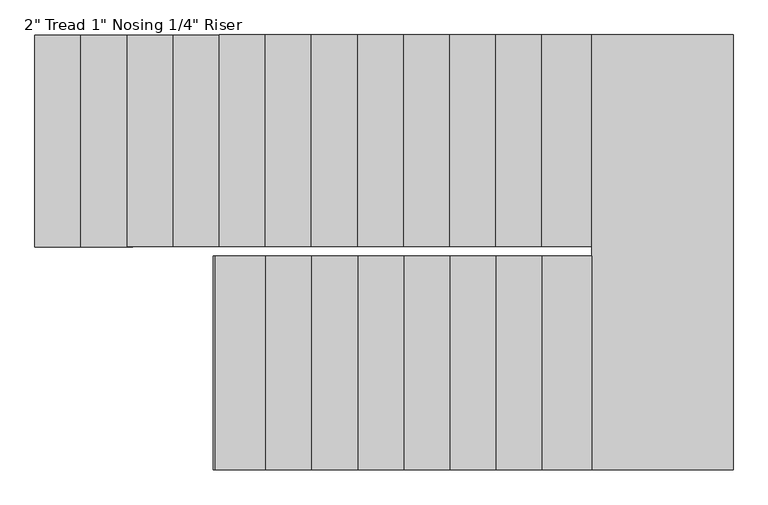
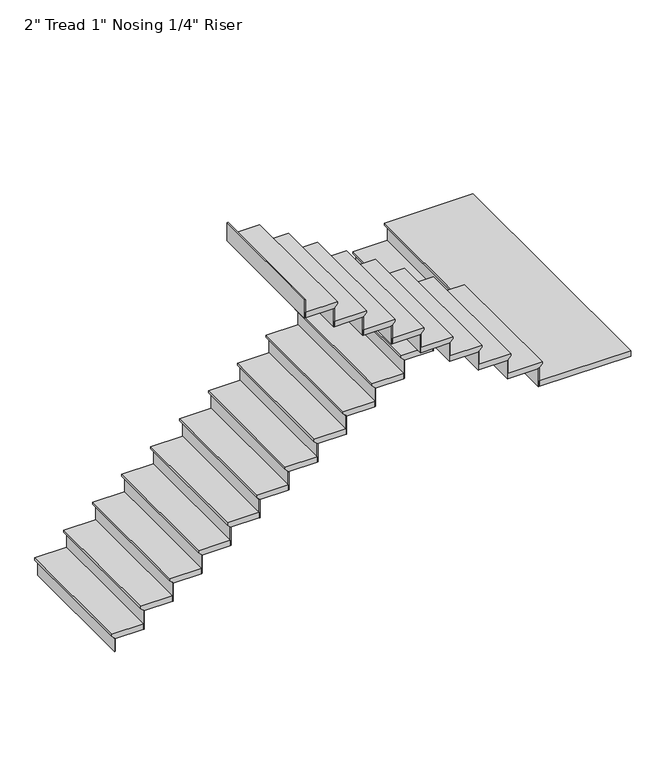
"""IFC4 building model written with IfcOpenShell, lengths in millimetres: stair flight geometry."""

from ifc_helpers import new_model, si_unit, origin, place, context, project, spatial, faceted_brep, source, transform, mapped, element, save


def stair_flight_20087966(model_context):
    return source(origin(), model_context, "Body", "Brep", [
        faceted_brep([(1811.8890963, 296.3962251, 150.2833333), (1811.8890963, 296.3962251, 169.3333333), (1811.8890963, 1464.7962251, 169.3333333), (1811.8890963, 1464.7962251, 150.2833333), (1837.2890963, 296.3962251, 124.8833333), (1837.2890963, 1464.7962251, 124.8833333), (2091.2890963, 296.3962251, 169.3333333), (2091.2890963, 1464.7962251, 169.3333333), (1837.2890963, 1464.7962251, 118.5333333), (2091.2890963, 1464.7962251, 118.5333333), (2091.2890963, 296.3962251, 118.5333333), (1837.2890963, 296.3962251, 118.5333333)], [[[0, 1, 2, 3]], [[4, 0, 3, 5]], [[2, 1, 6, 7]], [[8, 9, 10, 11]], [[2, 7, 9, 8, 5, 3]], [[8, 11, 4, 5]], [[6, 1, 0, 4, 11, 10]], [[7, 6, 10, 9]]]),
        faceted_brep([(1837.2890963, 296.3962251, 118.5333333), (1837.2890963, 296.3962251, 0.0), (1843.6390963, 296.3962251, 0.0), (1843.6390963, 296.3962251, 118.5333333), (1837.2890963, 1464.7962251, 118.5333333), (1843.6390963, 1464.7962251, 118.5333333), (1843.6390963, 1464.7962251, 0.0), (1837.2890963, 1464.7962251, 0.0)], [[[0, 1, 2, 3]], [[4, 5, 6, 7]], [[1, 0, 4, 7]], [[2, 1, 7, 6]], [[3, 2, 6, 5]], [[0, 3, 5, 4]]]),
        faceted_brep([(2091.2890963, 296.3962251, 287.8666667), (2091.2890963, 296.3962251, 118.5333333), (2097.6390963, 296.3962251, 118.5333333), (2097.6390963, 296.3962251, 287.8666667), (2091.2890963, 1464.7962251, 287.8666667), (2097.6390963, 1464.7962251, 287.8666667), (2097.6390963, 1464.7962251, 118.5333333), (2091.2890963, 1464.7962251, 118.5333333)], [[[0, 1, 2, 3]], [[4, 5, 6, 7]], [[1, 0, 4, 7]], [[2, 1, 7, 6]], [[3, 2, 6, 5]], [[0, 3, 5, 4]]]),
        faceted_brep([(2065.8890963, 1464.7962251, 338.6666667), (2065.8890963, 296.3962251, 338.6666667), (2345.2890963, 296.3962251, 338.6666667), (2345.2890963, 1464.7962251, 338.6666667), (2091.2890963, 1464.7962251, 287.8666667), (2345.2890963, 1464.7962251, 287.8666667), (2345.2890963, 296.3962251, 287.8666667), (2091.2890963, 296.3962251, 287.8666667), (2091.2890963, 1464.7962251, 294.2166667), (2065.8890963, 1464.7962251, 319.6166667), (2091.2890963, 296.3962251, 294.2166667), (2065.8890963, 296.3962251, 319.6166667)], [[[0, 1, 2, 3]], [[4, 5, 6, 7]], [[0, 3, 5, 4, 8, 9]], [[4, 7, 10, 8]], [[2, 1, 11, 10, 7, 6]], [[3, 2, 6, 5]], [[11, 1, 0, 9]], [[10, 11, 9, 8]]]),
        faceted_brep([(2345.2890963, 296.3962251, 457.2), (2345.2890963, 296.3962251, 287.8666667), (2351.6390963, 296.3962251, 287.8666667), (2351.6390963, 296.3962251, 457.2), (2345.2890963, 1464.7962251, 457.2), (2351.6390963, 1464.7962251, 457.2), (2351.6390963, 1464.7962251, 287.8666667), (2345.2890963, 1464.7962251, 287.8666667)], [[[0, 1, 2, 3]], [[4, 5, 6, 7]], [[1, 0, 4, 7]], [[2, 1, 7, 6]], [[3, 2, 6, 5]], [[0, 3, 5, 4]]]),
        faceted_brep([(2319.8890963, 1464.7962251, 508.0), (2319.8890963, 296.3962251, 508.0), (2599.2890963, 296.3962251, 508.0), (2599.2890963, 1464.7962251, 508.0), (2345.2890963, 1464.7962251, 457.2), (2599.2890963, 1464.7962251, 457.2), (2599.2890963, 296.3962251, 457.2), (2345.2890963, 296.3962251, 457.2), (2345.2890963, 1464.7962251, 463.55), (2319.8890963, 1464.7962251, 488.95), (2345.2890963, 296.3962251, 463.55), (2319.8890963, 296.3962251, 488.95)], [[[0, 1, 2, 3]], [[4, 5, 6, 7]], [[0, 3, 5, 4, 8, 9]], [[4, 7, 10, 8]], [[2, 1, 11, 10, 7, 6]], [[3, 2, 6, 5]], [[11, 1, 0, 9]], [[10, 11, 9, 8]]]),
        faceted_brep([(2599.2890963, 296.3962251, 626.5333333), (2599.2890963, 296.3962251, 457.2), (2605.6390963, 296.3962251, 457.2), (2605.6390963, 296.3962251, 626.5333333), (2599.2890963, 1464.7962251, 626.5333333), (2605.6390963, 1464.7962251, 626.5333333), (2605.6390963, 1464.7962251, 457.2), (2599.2890963, 1464.7962251, 457.2)], [[[0, 1, 2, 3]], [[4, 5, 6, 7]], [[1, 0, 4, 7]], [[2, 1, 7, 6]], [[3, 2, 6, 5]], [[0, 3, 5, 4]]]),
        faceted_brep([(2573.8890963, 1464.7962251, 677.3333333), (2573.8890963, 296.3962251, 677.3333333), (2853.2890963, 296.3962251, 677.3333333), (2853.2890963, 1464.7962251, 677.3333333), (2599.2890963, 1464.7962251, 626.5333333), (2853.2890963, 1464.7962251, 626.5333333), (2853.2890963, 296.3962251, 626.5333333), (2599.2890963, 296.3962251, 626.5333333), (2599.2890963, 1464.7962251, 632.8833333), (2573.8890963, 1464.7962251, 658.2833333), (2599.2890963, 296.3962251, 632.8833333), (2573.8890963, 296.3962251, 658.2833333)], [[[0, 1, 2, 3]], [[4, 5, 6, 7]], [[0, 3, 5, 4, 8, 9]], [[4, 7, 10, 8]], [[2, 1, 11, 10, 7, 6]], [[3, 2, 6, 5]], [[11, 1, 0, 9]], [[10, 11, 9, 8]]]),
        faceted_brep([(2853.2890963, 296.3962251, 795.8666667), (2853.2890963, 296.3962251, 626.5333333), (2859.6390963, 296.3962251, 626.5333333), (2859.6390963, 296.3962251, 795.8666667), (2853.2890963, 1464.7962251, 795.8666667), (2859.6390963, 1464.7962251, 795.8666667), (2859.6390963, 1464.7962251, 626.5333333), (2853.2890963, 1464.7962251, 626.5333333)], [[[0, 1, 2, 3]], [[4, 5, 6, 7]], [[1, 0, 4, 7]], [[2, 1, 7, 6]], [[3, 2, 6, 5]], [[0, 3, 5, 4]]]),
        faceted_brep([(2827.8890963, 1464.7962251, 846.6666667), (2827.8890963, 296.3962251, 846.6666667), (3107.2890963, 296.3962251, 846.6666667), (3107.2890963, 1464.7962251, 846.6666667), (2853.2890963, 1464.7962251, 795.8666667), (3107.2890963, 1464.7962251, 795.8666667), (3107.2890963, 296.3962251, 795.8666667), (2853.2890963, 296.3962251, 795.8666667), (2853.2890963, 1464.7962251, 802.2166667), (2827.8890963, 1464.7962251, 827.6166667), (2853.2890963, 296.3962251, 802.2166667), (2827.8890963, 296.3962251, 827.6166667)], [[[0, 1, 2, 3]], [[4, 5, 6, 7]], [[0, 3, 5, 4, 8, 9]], [[4, 7, 10, 8]], [[2, 1, 11, 10, 7, 6]], [[3, 2, 6, 5]], [[11, 1, 0, 9]], [[10, 11, 9, 8]]]),
        faceted_brep([(3107.2890963, 296.3962251, 965.2), (3107.2890963, 296.3962251, 795.8666667), (3113.6390963, 296.3962251, 795.8666667), (3113.6390963, 296.3962251, 965.2), (3107.2890963, 1464.7962251, 965.2), (3113.6390963, 1464.7962251, 965.2), (3113.6390963, 1464.7962251, 795.8666667), (3107.2890963, 1464.7962251, 795.8666667)], [[[0, 1, 2, 3]], [[4, 5, 6, 7]], [[1, 0, 4, 7]], [[2, 1, 7, 6]], [[3, 2, 6, 5]], [[0, 3, 5, 4]]]),
        faceted_brep([(3081.8890963, 1464.7962251, 1016.0), (3081.8890963, 296.3962251, 1016.0), (3361.2890963, 296.3962251, 1016.0), (3361.2890963, 1464.7962251, 1016.0), (3107.2890963, 1464.7962251, 965.2), (3361.2890963, 1464.7962251, 965.2), (3361.2890963, 296.3962251, 965.2), (3107.2890963, 296.3962251, 965.2), (3107.2890963, 1464.7962251, 971.55), (3081.8890963, 1464.7962251, 996.95), (3107.2890963, 296.3962251, 971.55), (3081.8890963, 296.3962251, 996.95)], [[[0, 1, 2, 3]], [[4, 5, 6, 7]], [[0, 3, 5, 4, 8, 9]], [[4, 7, 10, 8]], [[2, 1, 11, 10, 7, 6]], [[3, 2, 6, 5]], [[11, 1, 0, 9]], [[10, 11, 9, 8]]]),
        faceted_brep([(3361.2890963, 296.3962251, 1134.5333333), (3361.2890963, 296.3962251, 965.2), (3367.6390963, 296.3962251, 965.2), (3367.6390963, 296.3962251, 1134.5333333), (3361.2890963, 1464.7962251, 1134.5333333), (3367.6390963, 1464.7962251, 1134.5333333), (3367.6390963, 1464.7962251, 965.2), (3361.2890963, 1464.7962251, 965.2)], [[[0, 1, 2, 3]], [[4, 5, 6, 7]], [[1, 0, 4, 7]], [[2, 1, 7, 6]], [[3, 2, 6, 5]], [[0, 3, 5, 4]]]),
        faceted_brep([(3335.8890963, 1464.7962251, 1185.3333333), (3335.8890963, 296.3962251, 1185.3333333), (3615.2890963, 296.3962251, 1185.3333333), (3615.2890963, 1464.7962251, 1185.3333333), (3361.2890963, 1464.7962251, 1134.5333333), (3615.2890963, 1464.7962251, 1134.5333333), (3615.2890963, 296.3962251, 1134.5333333), (3361.2890963, 296.3962251, 1134.5333333), (3361.2890963, 1464.7962251, 1140.8833333), (3335.8890963, 1464.7962251, 1166.2833333), (3361.2890963, 296.3962251, 1140.8833333), (3335.8890963, 296.3962251, 1166.2833333)], [[[0, 1, 2, 3]], [[4, 5, 6, 7]], [[0, 3, 5, 4, 8, 9]], [[4, 7, 10, 8]], [[2, 1, 11, 10, 7, 6]], [[3, 2, 6, 5]], [[11, 1, 0, 9]], [[10, 11, 9, 8]]]),
        faceted_brep([(3615.2890963, 296.3962251, 1303.8666667), (3615.2890963, 296.3962251, 1134.5333333), (3621.6390963, 296.3962251, 1134.5333333), (3621.6390963, 296.3962251, 1303.8666667), (3615.2890963, 1464.7962251, 1303.8666667), (3621.6390963, 1464.7962251, 1303.8666667), (3621.6390963, 1464.7962251, 1134.5333333), (3615.2890963, 1464.7962251, 1134.5333333)], [[[0, 1, 2, 3]], [[4, 5, 6, 7]], [[1, 0, 4, 7]], [[2, 1, 7, 6]], [[3, 2, 6, 5]], [[0, 3, 5, 4]]]),
        faceted_brep([(3589.8890963, 1464.7962251, 1354.6666667), (3589.8890963, 296.3962251, 1354.6666667), (3869.2890963, 296.3962251, 1354.6666667), (3869.2890963, 1464.7962251, 1354.6666667), (3615.2890963, 1464.7962251, 1303.8666667), (3869.2890963, 1464.7962251, 1303.8666667), (3869.2890963, 296.3962251, 1303.8666667), (3615.2890963, 296.3962251, 1303.8666667), (3615.2890963, 1464.7962251, 1310.2166667), (3589.8890963, 1464.7962251, 1335.6166667), (3615.2890963, 296.3962251, 1310.2166667), (3589.8890963, 296.3962251, 1335.6166667)], [[[0, 1, 2, 3]], [[4, 5, 6, 7]], [[0, 3, 5, 4, 8, 9]], [[4, 7, 10, 8]], [[2, 1, 11, 10, 7, 6]], [[3, 2, 6, 5]], [[11, 1, 0, 9]], [[10, 11, 9, 8]]]),
        faceted_brep([(3869.2890963, 296.3962251, 1473.2), (3869.2890963, 296.3962251, 1303.8666667), (3875.6390963, 296.3962251, 1303.8666667), (3875.6390963, 296.3962251, 1473.2), (3869.2890963, 1464.7962251, 1473.2), (3875.6390963, 1464.7962251, 1473.2), (3875.6390963, 1464.7962251, 1303.8666667), (3869.2890963, 1464.7962251, 1303.8666667)], [[[0, 1, 2, 3]], [[4, 5, 6, 7]], [[1, 0, 4, 7]], [[2, 1, 7, 6]], [[3, 2, 6, 5]], [[0, 3, 5, 4]]]),
        faceted_brep([(3843.8890963, 1464.7962251, 1524.0), (3843.8890963, 296.3962251, 1524.0), (4123.2890963, 296.3962251, 1524.0), (4123.2890963, 1464.7962251, 1524.0), (3869.2890963, 1464.7962251, 1473.2), (4123.2890963, 1464.7962251, 1473.2), (4123.2890963, 296.3962251, 1473.2), (3869.2890963, 296.3962251, 1473.2), (3869.2890963, 1464.7962251, 1479.55), (3843.8890963, 1464.7962251, 1504.95), (3869.2890963, 296.3962251, 1479.55), (3843.8890963, 296.3962251, 1504.95)], [[[0, 1, 2, 3]], [[4, 5, 6, 7]], [[0, 3, 5, 4, 8, 9]], [[4, 7, 10, 8]], [[2, 1, 11, 10, 7, 6]], [[3, 2, 6, 5]], [[11, 1, 0, 9]], [[10, 11, 9, 8]]]),
        faceted_brep([(4123.2890963, 296.3962251, 1642.5333333), (4123.2890963, 296.3962251, 1473.2), (4129.6390963, 296.3962251, 1473.2), (4129.6390963, 296.3962251, 1642.5333333), (4123.2890963, 1464.7962251, 1642.5333333), (4129.6390963, 1464.7962251, 1642.5333333), (4129.6390963, 1464.7962251, 1473.2), (4123.2890963, 1464.7962251, 1473.2)], [[[0, 1, 2, 3]], [[4, 5, 6, 7]], [[1, 0, 4, 7]], [[2, 1, 7, 6]], [[3, 2, 6, 5]], [[0, 3, 5, 4]]]),
        faceted_brep([(4097.8890963, 1464.7962251, 1693.3333333), (4097.8890963, 296.3962251, 1693.3333333), (4377.2890963, 296.3962251, 1693.3333333), (4377.2890963, 1464.7962251, 1693.3333333), (4123.2890963, 1464.7962251, 1642.5333333), (4377.2890963, 1464.7962251, 1642.5333333), (4377.2890963, 296.3962251, 1642.5333333), (4123.2890963, 296.3962251, 1642.5333333), (4123.2890963, 1464.7962251, 1648.8833333), (4097.8890963, 1464.7962251, 1674.2833333), (4123.2890963, 296.3962251, 1648.8833333), (4097.8890963, 296.3962251, 1674.2833333)], [[[0, 1, 2, 3]], [[4, 5, 6, 7]], [[0, 3, 5, 4, 8, 9]], [[4, 7, 10, 8]], [[2, 1, 11, 10, 7, 6]], [[3, 2, 6, 5]], [[11, 1, 0, 9]], [[10, 11, 9, 8]]]),
        faceted_brep([(4377.2890963, 296.3962251, 1811.8666667), (4377.2890963, 296.3962251, 1642.5333333), (4383.6390963, 296.3962251, 1642.5333333), (4383.6390963, 296.3962251, 1811.8666667), (4377.2890963, 1464.7962251, 1811.8666667), (4383.6390963, 1464.7962251, 1811.8666667), (4383.6390963, 1464.7962251, 1642.5333333), (4377.2890963, 1464.7962251, 1642.5333333)], [[[0, 1, 2, 3]], [[4, 5, 6, 7]], [[1, 0, 4, 7]], [[2, 1, 7, 6]], [[3, 2, 6, 5]], [[0, 3, 5, 4]]]),
        faceted_brep([(4351.8890963, 1464.7962251, 1862.6666667), (4351.8890963, 296.3962251, 1862.6666667), (4631.2890963, 296.3962251, 1862.6666667), (4631.2890963, 1464.7962251, 1862.6666667), (4377.2890963, 1464.7962251, 1811.8666667), (4631.2890963, 1464.7962251, 1811.8666667), (4631.2890963, 296.3962251, 1811.8666667), (4377.2890963, 296.3962251, 1811.8666667), (4377.2890963, 1464.7962251, 1818.2166667), (4351.8890963, 1464.7962251, 1843.6166667), (4377.2890963, 296.3962251, 1818.2166667), (4351.8890963, 296.3962251, 1843.6166667)], [[[0, 1, 2, 3]], [[4, 5, 6, 7]], [[0, 3, 5, 4, 8, 9]], [[4, 7, 10, 8]], [[2, 1, 11, 10, 7, 6]], [[3, 2, 6, 5]], [[11, 1, 0, 9]], [[10, 11, 9, 8]]]),
        faceted_brep([(4631.2890963, 296.3962251, 1981.2), (4631.2890963, 296.3962251, 1811.8666667), (4637.6390963, 296.3962251, 1811.8666667), (4637.6390963, 296.3962251, 1981.2), (4631.2890963, 1464.7962251, 1981.2), (4637.6390963, 1464.7962251, 1981.2), (4637.6390963, 1464.7962251, 1811.8666667), (4631.2890963, 1464.7962251, 1811.8666667)], [[[0, 1, 2, 3]], [[4, 5, 6, 7]], [[1, 0, 4, 7]], [[2, 1, 7, 6]], [[3, 2, 6, 5]], [[0, 3, 5, 4]]]),
        faceted_brep([(4605.8890963, 1464.7962251, 2032.0), (4605.8890963, 296.3962251, 2032.0), (4906.4326586, 296.3962251, 2032.0), (4906.4326586, 1464.7962251, 2032.0), (4631.2890963, 1464.7962251, 1981.2), (4906.4326586, 1464.7962251, 1981.2), (4906.4326586, 296.3962251, 1981.2), (4631.2890963, 296.3962251, 1981.2), (4631.2890963, 1464.7962251, 1987.55), (4605.8890963, 1464.7962251, 2012.95), (4631.2890963, 296.3962251, 1987.55), (4605.8890963, 296.3962251, 2012.95)], [[[0, 1, 2, 3]], [[4, 5, 6, 7]], [[0, 3, 5, 4, 8, 9]], [[4, 7, 10, 8]], [[2, 1, 11, 10, 7, 6]], [[3, 2, 6, 5]], [[11, 1, 0, 9]], [[10, 11, 9, 8]]]),
        faceted_brep([(4906.4326586, 296.3962251, 2150.5333333), (4906.4326586, 296.3962251, 1981.2), (4912.7826586, 296.3962251, 1981.2), (4912.7826586, 296.3962251, 2150.5333333), (4906.4326586, 1464.7962251, 2150.5333333), (4912.7826586, 1464.7962251, 2150.5333333), (4912.7826586, 1464.7962251, 1981.2), (4906.4326586, 1464.7962251, 1981.2)], [[[0, 1, 2, 3]], [[4, 5, 6, 7]], [[1, 0, 4, 7]], [[2, 1, 7, 6]], [[3, 2, 6, 5]], [[0, 3, 5, 4]]]),
        faceted_brep([(4855.6326586, -935.5037749, 2201.3333333), (5659.9890963, -935.5037749, 2201.3333333), (5659.9890963, 1464.7962251, 2201.3333333), (4881.0326586, 1464.7962251, 2201.3333333), (4881.0326586, 245.5962251, 2201.3333333), (4855.6326586, 245.5962251, 2201.3333333), (5659.9890963, -935.5037749, 2150.5333333), (4855.6326586, -935.5037749, 2150.5333333), (4855.6326586, 245.5962251, 2150.5333333), (4881.0326586, 245.5962251, 2150.5333333), (4881.0326586, 296.3962251, 2150.5333333), (4906.4326586, 296.3962251, 2150.5333333), (4906.4326586, 1464.7962251, 2150.5333333), (5659.9890963, 1464.7962251, 2150.5333333), (4906.4326586, 1464.7962251, 2156.8833333), (4881.0326586, 1464.7962251, 2182.2833333), (4906.4326586, 296.3962251, 2156.8833333), (4881.0326586, 296.3962251, 2182.2833333)], [[[0, 1, 2, 3, 4, 5]], [[6, 7, 8, 9, 10, 11, 12, 13]], [[1, 0, 7, 6]], [[2, 1, 6, 13]], [[3, 2, 13, 12, 14, 15]], [[12, 11, 16, 14]], [[11, 10, 17, 16]], [[4, 3, 15, 17, 10, 9]], [[5, 4, 9, 8]], [[0, 5, 8, 7]], [[15, 14, 16, 17]]]),
        faceted_brep([(4855.6326586, 245.5962251, 2319.8666667), (4855.6326586, 245.5962251, 2150.5333333), (4849.2826586, 245.5962251, 2150.5333333), (4849.2826586, 245.5962251, 2319.8666667), (4855.6326586, -935.5037749, 2319.8666667), (4849.2826586, -935.5037749, 2319.8666667), (4849.2826586, -935.5037749, 2150.5333333), (4855.6326586, -935.5037749, 2150.5333333)], [[[0, 1, 2, 3]], [[4, 5, 6, 7]], [[1, 0, 4, 7]], [[2, 1, 7, 6]], [[3, 2, 6, 5]], [[0, 3, 5, 4]]]),
        faceted_brep([(4881.0326586, -935.5037749, 2370.6666667), (4881.0326586, 245.5962251, 2370.6666667), (4580.4890963, 245.5962251, 2370.6666667), (4580.4890963, -935.5037749, 2370.6666667), (4855.6326586, -935.5037749, 2319.8666667), (4580.4890963, -935.5037749, 2319.8666667), (4580.4890963, 245.5962251, 2319.8666667), (4855.6326586, 245.5962251, 2319.8666667), (4855.6326586, -935.5037749, 2326.2166667), (4881.0326586, -935.5037749, 2351.6166667), (4855.6326586, 245.5962251, 2326.2166667), (4881.0326586, 245.5962251, 2351.6166667)], [[[0, 1, 2, 3]], [[4, 5, 6, 7]], [[0, 3, 5, 4, 8, 9]], [[4, 7, 10, 8]], [[2, 1, 11, 10, 7, 6]], [[3, 2, 6, 5]], [[11, 1, 0, 9]], [[10, 11, 9, 8]]]),
        faceted_brep([(4580.4890963, 245.5962251, 2489.2), (4580.4890963, 245.5962251, 2319.8666667), (4574.1390963, 245.5962251, 2319.8666667), (4574.1390963, 245.5962251, 2489.2), (4580.4890963, -935.5037749, 2489.2), (4574.1390963, -935.5037749, 2489.2), (4574.1390963, -935.5037749, 2319.8666667), (4580.4890963, -935.5037749, 2319.8666667)], [[[0, 1, 2, 3]], [[4, 5, 6, 7]], [[1, 0, 4, 7]], [[2, 1, 7, 6]], [[3, 2, 6, 5]], [[0, 3, 5, 4]]]),
        faceted_brep([(4605.8890963, -935.5037749, 2540.0), (4605.8890963, 245.5962251, 2540.0), (4326.4890963, 245.5962251, 2540.0), (4326.4890963, -935.5037749, 2540.0), (4580.4890963, -935.5037749, 2489.2), (4326.4890963, -935.5037749, 2489.2), (4326.4890963, 245.5962251, 2489.2), (4580.4890963, 245.5962251, 2489.2), (4580.4890963, -935.5037749, 2495.55), (4605.8890963, -935.5037749, 2520.95), (4580.4890963, 245.5962251, 2495.55), (4605.8890963, 245.5962251, 2520.95)], [[[0, 1, 2, 3]], [[4, 5, 6, 7]], [[0, 3, 5, 4, 8, 9]], [[4, 7, 10, 8]], [[2, 1, 11, 10, 7, 6]], [[3, 2, 6, 5]], [[11, 1, 0, 9]], [[10, 11, 9, 8]]]),
        faceted_brep([(4326.4890963, 245.5962251, 2658.5333333), (4326.4890963, 245.5962251, 2489.2), (4320.1390963, 245.5962251, 2489.2), (4320.1390963, 245.5962251, 2658.5333333), (4326.4890963, -935.5037749, 2658.5333333), (4320.1390963, -935.5037749, 2658.5333333), (4320.1390963, -935.5037749, 2489.2), (4326.4890963, -935.5037749, 2489.2)], [[[0, 1, 2, 3]], [[4, 5, 6, 7]], [[1, 0, 4, 7]], [[2, 1, 7, 6]], [[3, 2, 6, 5]], [[0, 3, 5, 4]]]),
        faceted_brep([(4351.8890963, -935.5037749, 2709.3333333), (4351.8890963, 245.5962251, 2709.3333333), (4072.4890963, 245.5962251, 2709.3333333), (4072.4890963, -935.5037749, 2709.3333333), (4326.4890963, -935.5037749, 2658.5333333), (4072.4890963, -935.5037749, 2658.5333333), (4072.4890963, 245.5962251, 2658.5333333), (4326.4890963, 245.5962251, 2658.5333333), (4326.4890963, -935.5037749, 2664.8833333), (4351.8890963, -935.5037749, 2690.2833333), (4326.4890963, 245.5962251, 2664.8833333), (4351.8890963, 245.5962251, 2690.2833333)], [[[0, 1, 2, 3]], [[4, 5, 6, 7]], [[0, 3, 5, 4, 8, 9]], [[4, 7, 10, 8]], [[2, 1, 11, 10, 7, 6]], [[3, 2, 6, 5]], [[11, 1, 0, 9]], [[10, 11, 9, 8]]]),
        faceted_brep([(4072.4890963, 245.5962251, 2827.8666667), (4072.4890963, 245.5962251, 2658.5333333), (4066.1390963, 245.5962251, 2658.5333333), (4066.1390963, 245.5962251, 2827.8666667), (4072.4890963, -935.5037749, 2827.8666667), (4066.1390963, -935.5037749, 2827.8666667), (4066.1390963, -935.5037749, 2658.5333333), (4072.4890963, -935.5037749, 2658.5333333)], [[[0, 1, 2, 3]], [[4, 5, 6, 7]], [[1, 0, 4, 7]], [[2, 1, 7, 6]], [[3, 2, 6, 5]], [[0, 3, 5, 4]]]),
        faceted_brep([(4097.8890963, -935.5037749, 2878.6666667), (4097.8890963, 245.5962251, 2878.6666667), (3818.4890963, 245.5962251, 2878.6666667), (3818.4890963, -935.5037749, 2878.6666667), (4072.4890963, -935.5037749, 2827.8666667), (3818.4890963, -935.5037749, 2827.8666667), (3818.4890963, 245.5962251, 2827.8666667), (4072.4890963, 245.5962251, 2827.8666667), (4072.4890963, -935.5037749, 2834.2166667), (4097.8890963, -935.5037749, 2859.6166667), (4072.4890963, 245.5962251, 2834.2166667), (4097.8890963, 245.5962251, 2859.6166667)], [[[0, 1, 2, 3]], [[4, 5, 6, 7]], [[0, 3, 5, 4, 8, 9]], [[4, 7, 10, 8]], [[2, 1, 11, 10, 7, 6]], [[3, 2, 6, 5]], [[11, 1, 0, 9]], [[10, 11, 9, 8]]]),
        faceted_brep([(3818.4890963, 245.5962251, 2997.2), (3818.4890963, 245.5962251, 2827.8666667), (3812.1390963, 245.5962251, 2827.8666667), (3812.1390963, 245.5962251, 2997.2), (3818.4890963, -935.5037749, 2997.2), (3812.1390963, -935.5037749, 2997.2), (3812.1390963, -935.5037749, 2827.8666667), (3818.4890963, -935.5037749, 2827.8666667)], [[[0, 1, 2, 3]], [[4, 5, 6, 7]], [[1, 0, 4, 7]], [[2, 1, 7, 6]], [[3, 2, 6, 5]], [[0, 3, 5, 4]]]),
        faceted_brep([(3843.8890963, -935.5037749, 3048.0), (3843.8890963, 245.5962251, 3048.0), (3564.4890963, 245.5962251, 3048.0), (3564.4890963, -935.5037749, 3048.0), (3818.4890963, -935.5037749, 2997.2), (3564.4890963, -935.5037749, 2997.2), (3564.4890963, 245.5962251, 2997.2), (3818.4890963, 245.5962251, 2997.2), (3818.4890963, -935.5037749, 3003.55), (3843.8890963, -935.5037749, 3028.95), (3818.4890963, 245.5962251, 3003.55), (3843.8890963, 245.5962251, 3028.95)], [[[0, 1, 2, 3]], [[4, 5, 6, 7]], [[0, 3, 5, 4, 8, 9]], [[4, 7, 10, 8]], [[2, 1, 11, 10, 7, 6]], [[3, 2, 6, 5]], [[11, 1, 0, 9]], [[10, 11, 9, 8]]]),
        faceted_brep([(3564.4890963, 245.5962251, 3166.5333333), (3564.4890963, 245.5962251, 2997.2), (3558.1390963, 245.5962251, 2997.2), (3558.1390963, 245.5962251, 3166.5333333), (3564.4890963, -935.5037749, 3166.5333333), (3558.1390963, -935.5037749, 3166.5333333), (3558.1390963, -935.5037749, 2997.2), (3564.4890963, -935.5037749, 2997.2)], [[[0, 1, 2, 3]], [[4, 5, 6, 7]], [[1, 0, 4, 7]], [[2, 1, 7, 6]], [[3, 2, 6, 5]], [[0, 3, 5, 4]]]),
        faceted_brep([(3589.8890963, -935.5037749, 3217.3333333), (3589.8890963, 245.5962251, 3217.3333333), (3310.4890963, 245.5962251, 3217.3333333), (3310.4890963, -935.5037749, 3217.3333333), (3564.4890963, -935.5037749, 3166.5333333), (3310.4890963, -935.5037749, 3166.5333333), (3310.4890963, 245.5962251, 3166.5333333), (3564.4890963, 245.5962251, 3166.5333333), (3564.4890963, -935.5037749, 3172.8833333), (3589.8890963, -935.5037749, 3198.2833333), (3564.4890963, 245.5962251, 3172.8833333), (3589.8890963, 245.5962251, 3198.2833333)], [[[0, 1, 2, 3]], [[4, 5, 6, 7]], [[0, 3, 5, 4, 8, 9]], [[4, 7, 10, 8]], [[2, 1, 11, 10, 7, 6]], [[3, 2, 6, 5]], [[11, 1, 0, 9]], [[10, 11, 9, 8]]]),
        faceted_brep([(3310.4890963, 245.5962251, 3335.8666667), (3310.4890963, 245.5962251, 3166.5333333), (3304.1390963, 245.5962251, 3166.5333333), (3304.1390963, 245.5962251, 3335.8666667), (3310.4890963, -935.5037749, 3335.8666667), (3304.1390963, -935.5037749, 3335.8666667), (3304.1390963, -935.5037749, 3166.5333333), (3310.4890963, -935.5037749, 3166.5333333)], [[[0, 1, 2, 3]], [[4, 5, 6, 7]], [[1, 0, 4, 7]], [[2, 1, 7, 6]], [[3, 2, 6, 5]], [[0, 3, 5, 4]]]),
        faceted_brep([(3335.8890963, -935.5037749, 3386.6666667), (3335.8890963, 245.5962251, 3386.6666667), (3056.4890963, 245.5962251, 3386.6666667), (3056.4890963, -935.5037749, 3386.6666667), (3310.4890963, -935.5037749, 3335.8666667), (3056.4890963, -935.5037749, 3335.8666667), (3056.4890963, 245.5962251, 3335.8666667), (3310.4890963, 245.5962251, 3335.8666667), (3310.4890963, -935.5037749, 3342.2166667), (3335.8890963, -935.5037749, 3367.6166667), (3310.4890963, 245.5962251, 3342.2166667), (3335.8890963, 245.5962251, 3367.6166667)], [[[0, 1, 2, 3]], [[4, 5, 6, 7]], [[0, 3, 5, 4, 8, 9]], [[4, 7, 10, 8]], [[2, 1, 11, 10, 7, 6]], [[3, 2, 6, 5]], [[11, 1, 0, 9]], [[10, 11, 9, 8]]]),
        faceted_brep([(3056.4890963, 245.5962251, 3505.2), (3056.4890963, 245.5962251, 3335.8666667), (3050.1390963, 245.5962251, 3335.8666667), (3050.1390963, 245.5962251, 3505.2), (3056.4890963, -935.5037749, 3505.2), (3050.1390963, -935.5037749, 3505.2), (3050.1390963, -935.5037749, 3335.8666667), (3056.4890963, -935.5037749, 3335.8666667)], [[[0, 1, 2, 3]], [[4, 5, 6, 7]], [[1, 0, 4, 7]], [[2, 1, 7, 6]], [[3, 2, 6, 5]], [[0, 3, 5, 4]]]),
        faceted_brep([(2802.4890963, 245.5962251, 3674.5333333), (2802.4890963, 245.5962251, 3505.2), (2796.1390963, 245.5962251, 3505.2), (2796.1390963, 245.5962251, 3674.5333333), (2802.4890963, -935.5037749, 3674.5333333), (2796.1390963, -935.5037749, 3674.5333333), (2796.1390963, -935.5037749, 3505.2), (2802.4890963, -935.5037749, 3505.2)], [[[0, 1, 2, 3]], [[4, 5, 6, 7]], [[1, 0, 4, 7]], [[2, 1, 7, 6]], [[3, 2, 6, 5]], [[0, 3, 5, 4]]]),
        faceted_brep([(3081.8890963, -935.5037749, 3556.0), (3081.8890963, 245.5962251, 3556.0), (2802.4890963, 245.5962251, 3556.0), (2802.4890963, -935.5037749, 3556.0), (3056.4890963, -935.5037749, 3505.2), (2802.4890963, -935.5037749, 3505.2), (2802.4890963, 245.5962251, 3505.2), (3056.4890963, 245.5962251, 3505.2), (3056.4890963, -935.5037749, 3511.55), (3081.8890963, -935.5037749, 3536.95), (3056.4890963, 245.5962251, 3511.55), (3081.8890963, 245.5962251, 3536.95)], [[[0, 1, 2, 3]], [[4, 5, 6, 7]], [[0, 3, 5, 4, 8, 9]], [[4, 7, 10, 8]], [[2, 1, 11, 10, 7, 6]], [[3, 2, 6, 5]], [[11, 1, 0, 9]], [[10, 11, 9, 8]]]),
    ])


if __name__ == "__main__":
    model = new_model("IFC4")
    model_context = context("Model", 3, world=origin())
    ifc_project = project(units=[si_unit("LENGTHUNIT", "METRE", prefix="MILLI")], contexts=[model_context])
    site = spatial("IfcSite", under=ifc_project)
    building = spatial("IfcBuilding", under=site)
    placement = place(None, origin())
    stair_flight_shape = stair_flight_20087966(model_context)
    element("IfcStairFlight", 1, ObjectType="2\" Tread 1\" Nosing 1/4\" Riser", at=placement, inside=building, context=model_context, shape_type="MappedRepresentation", body=[
        mapped(stair_flight_shape, transform((0.0, 0.0, 0.0), x_axis=(1.0, 0.0, 0.0), y_axis=(0.0, 1.0, 0.0), z_axis=(0.0, 0.0, 1.0))),
    ])
    save(model, "model.ifc")
